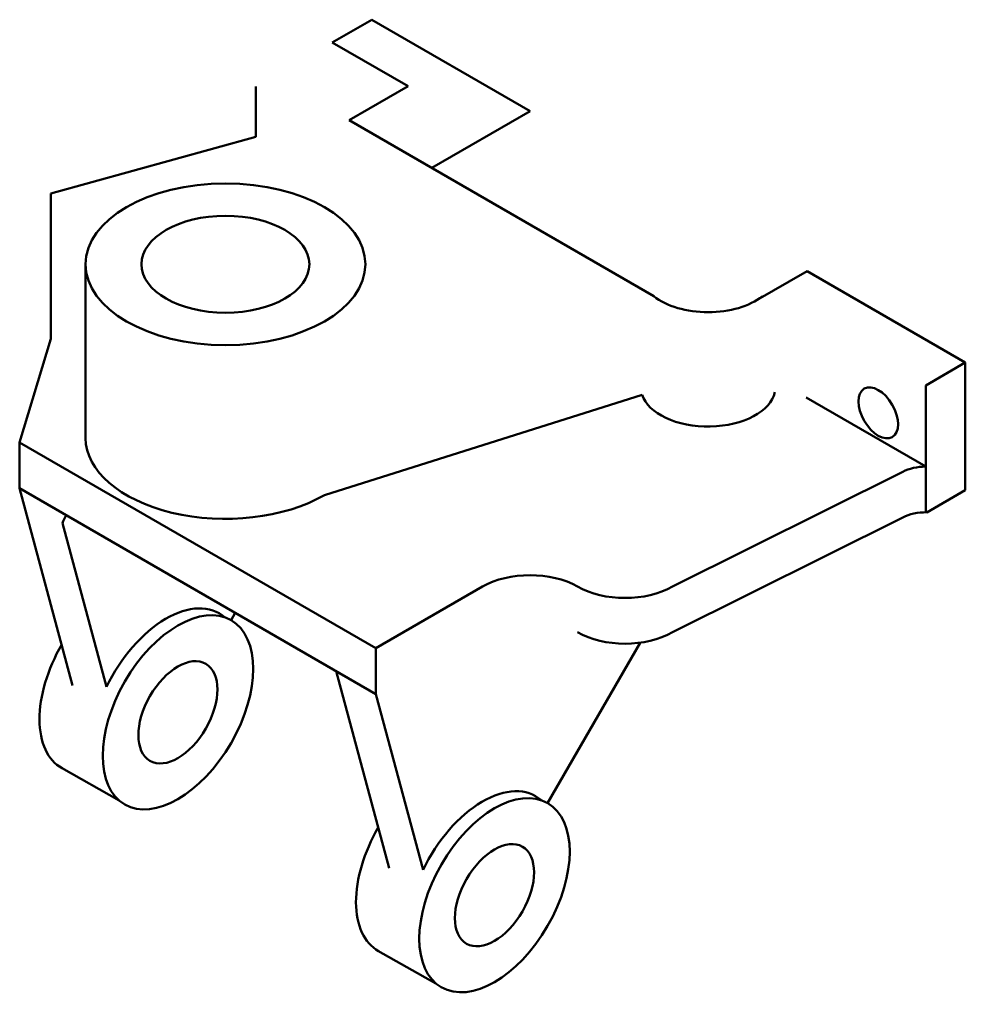
# Model space of a CAD drawing. Units: inches. Extents: x 1911 to 53588, y 1283 to 37932.
# Tile 1 of 2: x 1911 to 2118, y 1283 to 1498. Entities that reach past the tile are written whole.
import ezdxf

# ---------------------------------------------------------------- set-up
doc = ezdxf.new("R2010")
doc.units = ezdxf.units.IN
doc.header["$MEASUREMENT"] = 0
doc.layers.add('M-OUTL', color=7, linetype='Continuous', lineweight=50)

msp = doc.modelspace()

# ---------------------------------------------------------------- linework, layer by layer
at = {"layer": 'M-OUTL'}
for p, q in [((1988.51, 1498.38), (1979.85, 1493.38)), ((2023.15, 1478.38), (1988.51, 1498.38)), ((1979.85, 1493.38), (1996.44, 1483.8)), ((1963.15, 1483.73), (1963.15, 1472.74)), ((1996.44, 1483.8), (1983.57, 1476.37)), ((2023.15, 1478.38), (2001.62, 1465.95)), ((2050.25, 1437.88), (1983.57, 1476.37)), ((1963.15, 1472.74), (1918.23, 1460.34)), ((1918.23, 1460.34), (1918.23, 1428.6)), ((1925.85, 1406.88), (1925.85, 1444.88)), ((2083.77, 1443.38), (2072.51, 1436.88)), ((2118.41, 1423.38), (2083.77, 1443.38)), ((1918.23, 1428.6), (1911.43, 1405.88)), ((2109.75, 1418.38), (2118.41, 1423.38)), ((2118.41, 1423.38), (2118.41, 1401.38)), ((2109.75, 1406.38), (2109.75, 1418.38)), ((1978.12, 1394.38), (2047.66, 1416.35)), ((2109.75, 1400.62), (2083.56, 1415.74)), ((2109.75, 1390.62), (2109.75, 1406.38)), ((1989.38, 1360.88), (1911.43, 1405.88)), ((1911.43, 1405.88), (1911.43, 1395.88)), ((2118.41, 1395.48), (2118.41, 1401.38)), ((2054.33, 1374.38), (2104.74, 1399.48)), ((1911.43, 1395.88), (1989.38, 1350.88)), ((1911.43, 1395.88), (1923.02, 1352.78)), ((2109.99, 1390.62), (2118.41, 1395.48)), ((2054.33, 1364.38), (2104.74, 1389.48)), ((1920.79, 1388.28), (1930.43, 1352.43)), ((2012.76, 1374.38), (1989.38, 1360.88)), ((1957.71, 1367.03), (1958.63, 1368.63)), ((2026.99, 1327.03), (2047.24, 1362.11)), ((1989.38, 1350.88), (1989.38, 1360.88)), ((1980.71, 1355.88), (1992.31, 1312.78)), ((1989.38, 1350.88), (1999.72, 1312.43)), ((1920.58, 1334.72), (1933.21, 1327.6)), ((1989.86, 1294.72), (2002.49, 1287.6))]:
    msp.add_line(p, q, dxfattribs=at)
for centre, major_axis in [((1956.47, 1444.88), (-30.62, 0)), ((1956.47, 1444.88), (-18.37, 0)), ((2099.36, 1412.38), (3.06, -5.3)), ((1946.07, 1346.88), (-11.64, -20.15)), ((1946.07, 1346.88), (-6.12, -10.61)), ((2015.36, 1306.88), (-11.64, -20.15)), ((2015.36, 1306.88), (-6.12, -10.61))]:
    msp.add_ellipse(centre, major_axis=major_axis, ratio=0.57735, dxfattribs=at)
for centre, major_axis, start_param, end_param in [((2062.12, 1442.88), (-14.7, 0), 0.630137, 2.511455), ((2062.12, 1432.88), (-14.7, 0), 3.759543, 3.77173), ((2062.12, 1417.88), (-14.7, 0), 0.180461, 3.023586), ((1956.47, 1406.88), (-30.62, 0), 0, 2.356194), ((2109.75, 1396.38), (-7.35, 0), 4.712389, 5.462182), ((1925.29, 1387.88), (-3.67, -6.36), 4.712389, 4.973596), ((2109.75, 1386.38), (-7.35, 0), 4.680317, 5.462182), ((2023.15, 1368.38), (-14.7, 0), 3.926991, 5.497787), ((2043.93, 1380.38), (-14.7, 0), 0.785398, 2.356194), ((1943.48, 1348.38), (-11.64, -20.15), 9.312896, 11.125309), ((2043.93, 1370.38), (-14.7, 0), 0.785398, 2.356194), ((1932.22, 1354.88), (-11.64, -20.15), 4.708243, 6.294771), ((2012.76, 1308.38), (-11.64, -20.15), 9.312896, 11.125309), ((2001.5, 1314.88), (-11.64, -20.15), 4.708243, 6.294771)]:
    msp.add_ellipse(centre, major_axis=major_axis, ratio=0.57735, start_param=start_param, end_param=end_param, dxfattribs=at)

doc.saveas('drawing.dxf')
